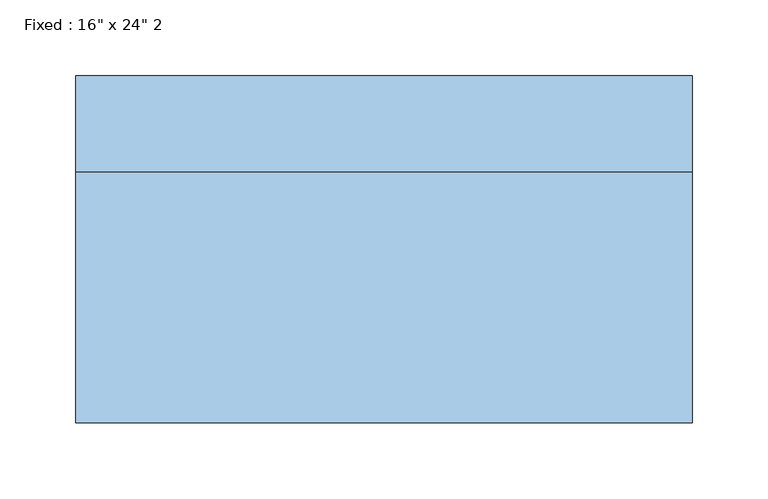
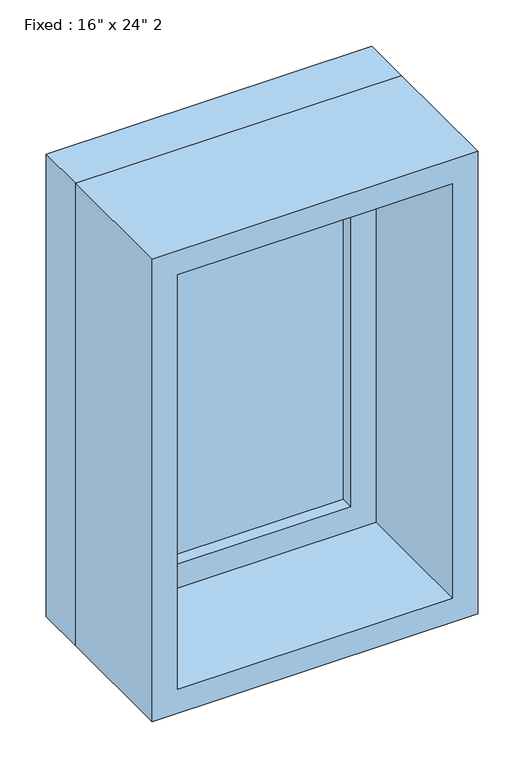
"""IFC4 building model written with IfcOpenShell, lengths in millimetres: window geometry."""

from ifc_helpers import new_model, si_unit, frame, origin, place, context, project, spatial, polyline, outline, extrude, source, transform, mapped, element, save


def window_aa618e30(model_context):
    return source(origin(), model_context, "Body", "SweptSolid", [
        extrude(outline(polyline([(101.6, 66.675), (-177.8, 66.675), (-177.8, 79.375), (101.6, 79.375), (101.6, 66.675)])), frame((0.0, 0.0, 977.9), z_axis=(0.0, 0.0, 1.0), x_axis=(1.0, 0.0, 0.0)), (0.0, 0.0, 1.0), 482.6),
        extrude(outline(polyline([(1504.95, -222.25), (933.45, -222.25), (933.45, 146.05), (1504.95, 146.05), (1504.95, -222.25)]), holes=[polyline([(1460.5, -177.8), (1460.5, 101.6), (977.9, 101.6), (977.9, -177.8), (1460.5, -177.8)])]), frame((0.0, 50.8, 0.0), z_axis=(0.0, 1.0, 0.0), x_axis=(0.0, 0.0, 1.0)), (0.0, 0.0, 1.0), 44.45),
        extrude(outline(polyline([(1524.0, -241.3), (914.4, -241.3), (914.4, 165.1), (1524.0, 165.1), (1524.0, -241.3)]), holes=[polyline([(1492.25, -209.55), (1492.25, 133.35), (946.15, 133.35), (946.15, -209.55), (1492.25, -209.55)])]), frame((0.0, -114.3, 0.0), z_axis=(0.0, 1.0, 0.0), x_axis=(0.0, 0.0, 1.0)), (0.0, 0.0, 1.0), 165.1),
        extrude(outline(polyline([(1524.0, 165.1), (1524.0, -241.3), (914.4, -241.3), (914.4, 165.1), (1524.0, 165.1)]), holes=[polyline([(1504.95, 146.05), (933.45, 146.05), (933.45, -222.25), (1504.95, -222.25), (1504.95, 146.05)])]), frame((0.0, 50.8, 0.0), z_axis=(0.0, 1.0, 0.0), x_axis=(0.0, 0.0, 1.0)), (0.0, 0.0, 1.0), 63.5),
    ])


if __name__ == "__main__":
    model = new_model("IFC4")
    model_context = context("Model", 3, world=origin())
    ifc_project = project(units=[si_unit("LENGTHUNIT", "METRE", prefix="MILLI")], contexts=[model_context])
    site = spatial("IfcSite", under=ifc_project)
    building = spatial("IfcBuilding", under=site)
    placement = place(None, origin())
    window_shape = window_aa618e30(model_context)
    element("IfcWindow", 1, ObjectType="Fixed : 16\" x 24\" 2", at=placement, inside=building, context=model_context, shape_type="MappedRepresentation", body=[
        mapped(window_shape, transform((0.0, 0.0, 0.0), x_axis=(1.0, 0.0, 0.0), y_axis=(0.0, 1.0, 0.0), z_axis=(0.0, 0.0, 1.0))),
    ])
    save(model, "model.ifc")

# Revit data of these elements
# Type "Fixed : 16\" x 24\" 2"
#   Type Mark = "21"
#   Construction Type Id = "GSP4R"
#   Assembly Code = "B2020100"
#   Analytic Construction = "1/8 in Pilkington single glazing"
#   Visual Light Transmittance = 0.9
#   Solar Heat Gain Coefficient = 0.78
#   Heat Transfer Coefficient (U) = 0.6496 BTU/(h·ft²·°F)
#   Height = 2' - 0"
#   Default Sill Height = 3' - 0"
#   Width = 1' - 4"
#   Window Inset = 0' - 0 3/4"
#   Define Thermal Properties by = 1
#   Glass Pane Material = Glass
#   Sash Material = Sash
#   Wall Closure = (empty or 0)
# Element 1 (IfcWindow, "Fixed : 16\" x 24\" 2")
#   Materials on its faces: "Sash", "Glass"
# Materials
#   "Glass": class "Glass", colour RGB 0 128 192, transparency 0.75, Description = "Soda Lime Glass", Cost = 0
#   "Sash": class "Wood", colour RGB 224 178 126, transparency 0, Cost = 0
